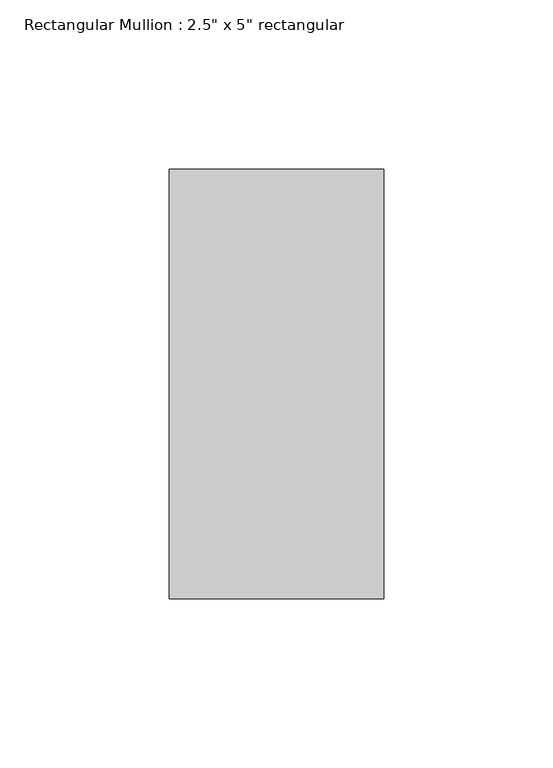
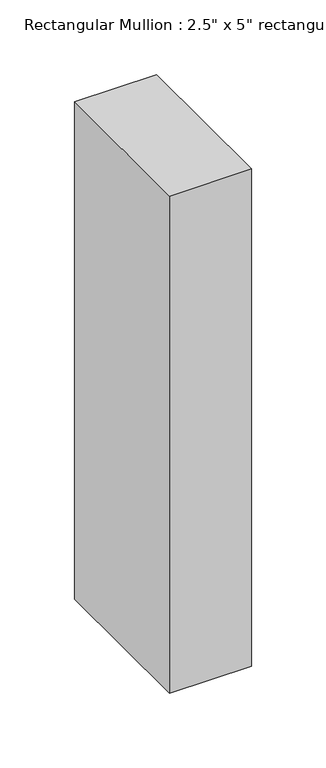
"""IFC4 building model written with IfcOpenShell, lengths in millimetres: member geometry."""

from ifc_helpers import new_model, si_unit, frame, origin, place, context, project, spatial, polyline, outline, extrude, source, transform, mapped, element, save


def member_7cfea1b5(model_context):
    return source(origin(), model_context, "Body", "SweptSolid", [
        extrude(outline(polyline([(0.0, 63.5), (0.0, -63.5), (-63.5, -63.5), (-63.5, 63.5), (0.0, 63.5)])), frame((0.0, 0.0, -406.4), z_axis=(0.0, 0.0, 1.0), x_axis=(1.0, 0.0, 0.0)), (0.0, 0.0, 1.0), 406.4),
    ])


if __name__ == "__main__":
    model = new_model("IFC4")
    model_context = context("Model", 3, world=origin())
    ifc_project = project(units=[si_unit("LENGTHUNIT", "METRE", prefix="MILLI")], contexts=[model_context])
    site = spatial("IfcSite", under=ifc_project)
    building = spatial("IfcBuilding", under=site)
    placement = place(None, origin())
    member_shape = member_7cfea1b5(model_context)
    element("IfcMember", 1, ObjectType="Rectangular Mullion : 2.5\" x 5\" rectangular", at=placement, inside=building, context=model_context, shape_type="MappedRepresentation", body=[
        mapped(member_shape, transform((0.0, 0.0, 0.0), x_axis=(1.0, 0.0, 0.0), y_axis=(0.0, 1.0, 0.0), z_axis=(0.0, 0.0, 1.0))),
    ])
    save(model, "model.ifc")

# Revit data of these elements
# Type "Rectangular Mullion : 2.5\" x 5\" rectangular"
#   built-in parameter 1007304 = 0.416667 (stored number, unit not read)
#   built-in parameter 1007301 = 0.104167 (stored number, unit not read)
#   built-in parameter 1007300 = 0.104167 (stored number, unit not read)
# Element 1 (IfcMember, "Rectangular Mullion : 2.5\" x 5\" rectangular")
#   Materials on its faces: "Door - Frame"
# Materials
#   "Door - Frame": colour RGB 118 70 51, transparency 0, Cost = 0
